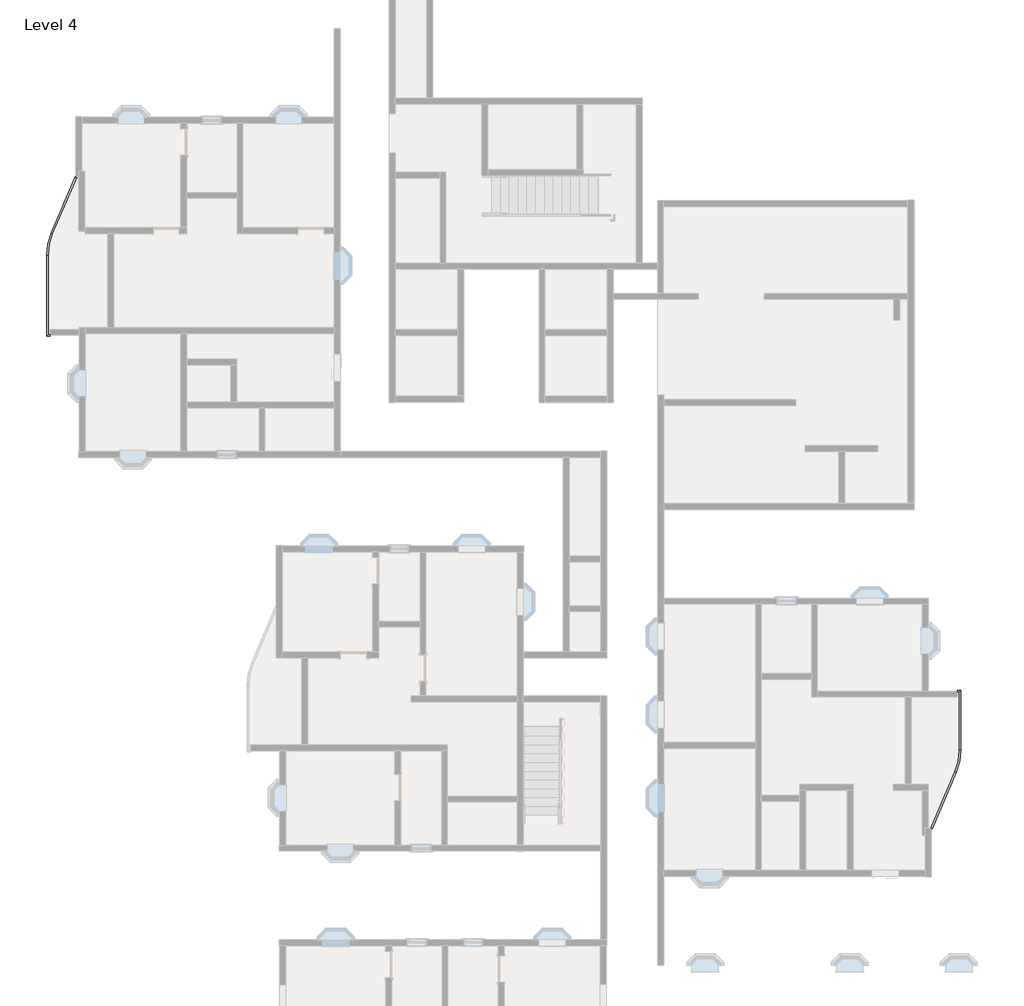
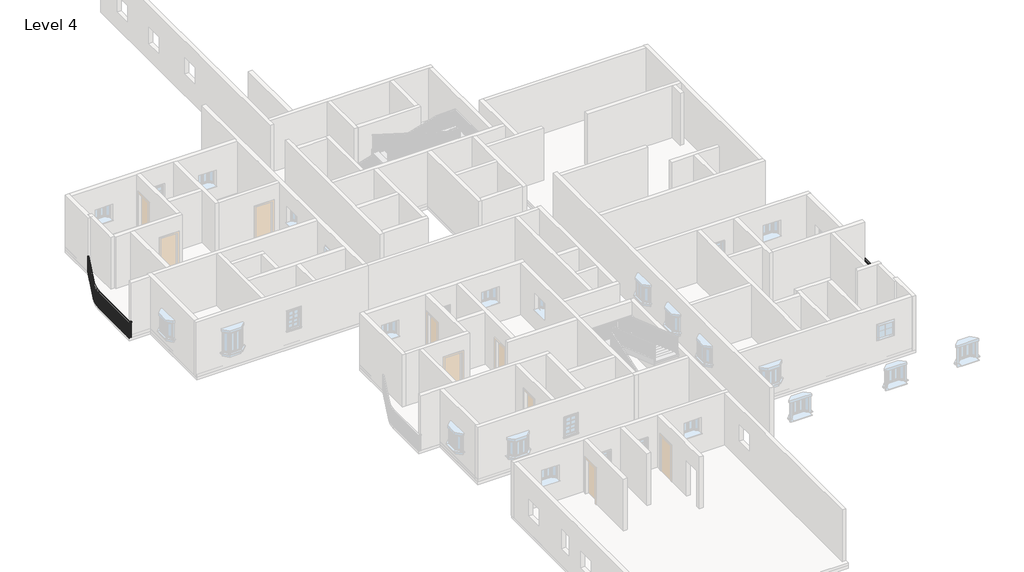
# One storey, part 9 of 14: 2 railings.
"""IFC4 building model written with IfcOpenShell, lengths in millimetres."""

from ifc_helpers import new_model, si_unit, frame, origin, place, context, project, spatial, polyline, circle_curve, outline, extrude, element, save
from ifc_brep_helpers import plane_surface, cylinder_surface, revolved_surface, advanced_brep

model = new_model("IFC4")

# Units and contexts
model_context = context("Model", 3, world=origin())
ifc_project = project(units=[si_unit("LENGTHUNIT", "METRE", prefix="MILLI")], contexts=[model_context])

# Site, building, storey
site = spatial("IfcSite", under=ifc_project)
building = spatial("IfcBuilding", under=site)
storey = spatial("IfcBuildingStorey", under=building, Name="Level 4", Elevation=9144.0)

# Railings
placement = place(None, origin())
element("IfcRailing", 1, ObjectType="Handrail - Rectangular", at=placement, inside=storey, context=model_context, shape_type="SolidModel", body=[
    advanced_brep(
    [(-19327.739878, 12446.0257339, 10058.4), (-19327.739878, 12446.0257339, 10007.6), (-19374.4383922, 12466.022953, 10007.6), (-19374.4383922, 12466.022953, 10058.4), (-20162.483418, 10496.6905323, 10058.4), (-20162.483418, 10496.6905323, 10007.6), (-20209.1819322, 10516.6877514, 10007.6), (-20209.1819322, 10516.6877514, 10058.4), (-20316.2891351, 9746.7948172, 10007.6), (-20316.2891351, 9746.7948172, 10058.4), (-20367.0891351, 9746.7948172, 10007.6), (-20367.0891351, 9746.7948172, 10058.4), (-20316.2891351, 7005.2583494, 10058.4), (-20316.2891351, 7005.2583494, 10007.6), (-20367.0891351, 6954.4583494, 10007.6), (-20367.0891351, 6954.4583494, 10058.4), (-20240.0891351, 7005.2583494, 10058.4), (-20240.0891351, 6954.4583494, 10058.4), (-20240.0891351, 6954.4583494, 10007.6), (-20240.0891351, 7005.2583494, 10007.6)],
    [
        (0, 1),
        (1, 2),
        (2, 3),
        (3, 0),
        (0, 4),
        (4, 5),
        (5, 1),
        (5, 6),
        (6, 2),
        (6, 7),
        (7, 3),
        (7, 4),
        (8, 5, circle_curve(frame((-18411.2891351, 9746.7948172, 10007.6), z_axis=(0.0, 0.0, -1.0), x_axis=(-0.919262090762392, 0.3936460446735823, 0.0)), 1905.0)),
        (4, 9, circle_curve(frame((-18411.2891351, 9746.7948172, 10058.4), z_axis=(0.0, 0.0, 1.0), x_axis=(-0.919262090762392, 0.3936460446735823, 0.0)), 1905.0)),
        (9, 8),
        (10, 6, circle_curve(frame((-18411.2891351, 9746.7948172, 10007.6), z_axis=(0.0, 0.0, -1.0), x_axis=(-0.919262090762392, 0.3936460446735823, 0.0)), 1955.8)),
        (8, 10),
        (11, 7, circle_curve(frame((-18411.2891351, 9746.7948172, 10058.4), z_axis=(0.0, 0.0, -1.0), x_axis=(-0.919262090762392, 0.3936460446735823, 0.0)), 1955.8)),
        (10, 11),
        (11, 9),
        (9, 12),
        (12, 13),
        (13, 8),
        (13, 14),
        (14, 10),
        (14, 15),
        (15, 11),
        (15, 12),
        (16, 17),
        (17, 18),
        (18, 19),
        (19, 16),
        (12, 16),
        (19, 13),
        (18, 14),
        (17, 15),
    ],
    [
        plane_surface(frame((-19351.0891351, 12456.0243434, 10058.4), z_axis=(0.3936460446735829, 0.9192620907623917, 0.0), x_axis=(0.9192620907623917, -0.3936460446735829, 0.0))),
        plane_surface(frame((-19327.739878, 12446.0257339, 10058.4), z_axis=(0.9192620907623915, -0.3936460446735834, 0.0), x_axis=(-0.3936460446735834, -0.9192620907623915, 0.0))),
        plane_surface(frame((-19327.739878, 12446.0257339, 10007.6), z_axis=(0.0, 0.0, -1.0000000000000002), x_axis=(-0.3936460446735834, -0.9192620907623915, 0.0))),
        plane_surface(frame((-19374.4383922, 12466.022953, 10007.6), z_axis=(-0.9192620907623916, 0.393646044673583, 0.0), x_axis=(-0.393646044673583, -0.9192620907623916, 0.0))),
        plane_surface(frame((-19374.4383922, 12466.022953, 10058.4), z_axis=(0.0, 0.0, 1.0), x_axis=(-0.393646044673583, -0.9192620907623916, 0.0))),
        revolved_surface(polyline([(-20162.483418002357, 10496.690532303173, 10058.4), (-20162.483418002357, 10496.690532303173, 10007.6)]), (-18411.2891351, 9746.7948172, 10058.4), (0.0, 0.0, 1.0)),
        plane_surface(frame((-18411.2891351, 9746.7948172, 10007.6), z_axis=(0.0, 0.0, -1.0), x_axis=(-0.919262090762392, 0.3936460446735823, 0.0))),
        cylinder_surface(frame((-18411.2891351, 9746.7948172, 10058.4), z_axis=(0.0, 0.0, 1.0), x_axis=(-0.919262090762392, 0.3936460446735823, 0.0)), 1955.8),
        plane_surface(frame((-18411.2891351, 9746.7948172, 10058.4), z_axis=(0.0, 0.0, 1.0), x_axis=(-0.919262090762392, 0.3936460446735823, 0.0))),
        plane_surface(frame((-20316.2891351, 9746.7948172, 10058.4), z_axis=(1.0, 0.0, 0.0), x_axis=(0.0, -1.0, 0.0))),
        plane_surface(frame((-20316.2891351, 9746.7948172, 10007.6), z_axis=(0.0, 0.0, -1.0), x_axis=(0.0, -1.0, 0.0))),
        plane_surface(frame((-20367.0891351, 9746.7948172, 10007.6), z_axis=(-1.0, 0.0, 0.0), x_axis=(0.0, -1.0, 0.0))),
        plane_surface(frame((-20367.0891351, 9746.7948172, 10058.4), z_axis=(0.0, 0.0, 1.0), x_axis=(0.0, -1.0, 0.0))),
        plane_surface(frame((-20240.0891351, 6979.8583494, 10058.4), z_axis=(1.0, 0.0, 0.0), x_axis=(0.0, 1.0, 0.0))),
        plane_surface(frame((-20316.2891351, 7005.2583494, 10058.4), z_axis=(0.0, 1.0, 0.0), x_axis=(1.0, 0.0, 0.0))),
        plane_surface(frame((-20316.2891351, 7005.2583494, 10007.6), z_axis=(0.0, 0.0, -1.0), x_axis=(1.0, 0.0, 0.0))),
        plane_surface(frame((-20367.0891351, 6954.4583494, 10007.6), z_axis=(0.0, -1.0, 0.0), x_axis=(1.0, 0.0, 0.0))),
        plane_surface(frame((-20367.0891351, 6954.4583494, 10058.4), z_axis=(0.0, 0.0, 1.0), x_axis=(1.0, 0.0, 0.0))),
    ],
    [
        (0, [[1, 2, 3, 4]]),
        (1, [[-1, 5, 6, 7]]),
        (2, [[-2, -7, 8, 9]]),
        (3, [[-3, -9, 10, 11]]),
        (4, [[-4, -11, 12, -5]]),
        (5, [[13, -6, 14, 15]]),
        (6, [[16, -8, -13, 17]]),
        (7, [[18, -10, -16, 19]]),
        (8, [[-14, -12, -18, 20]]),
        (9, [[-15, 21, 22, 23]]),
        (10, [[-17, -23, 24, 25]]),
        (11, [[-19, -25, 26, 27]]),
        (12, [[-20, -27, 28, -21]]),
        (13, [[29, 30, 31, 32]]),
        (14, [[-22, 33, -32, 34]]),
        (15, [[-24, -34, -31, 35]]),
        (16, [[-26, -35, -30, 36]]),
        (17, [[-28, -36, -29, -33]]),
    ],
),
    extrude(outline(polyline([(-20351.2141351, 7013.1198172), (-20332.1641351, 7013.1198172), (-20332.1641351, 6994.0698172), (-20351.2141351, 6994.0698172), (-20351.2141351, 7013.1198172)])), frame((0.0, 0.0, 9144.0), z_axis=(0.0, 0.0, 1.0), x_axis=(1.0, 0.0, 0.0)), (0.0, 0.0, 1.0), 863.6),
    extrude(outline(polyline([(-20351.2141351, 7114.7198172), (-20332.1641351, 7114.7198172), (-20332.1641351, 7095.6698172), (-20351.2141351, 7095.6698172), (-20351.2141351, 7114.7198172)])), frame((0.0, 0.0, 9144.0), z_axis=(0.0, 0.0, 1.0), x_axis=(1.0, 0.0, 0.0)), (0.0, 0.0, 1.0), 863.6),
    extrude(outline(polyline([(-20351.2141351, 7216.3198172), (-20332.1641351, 7216.3198172), (-20332.1641351, 7197.2698172), (-20351.2141351, 7197.2698172), (-20351.2141351, 7216.3198172)])), frame((0.0, 0.0, 9144.0), z_axis=(0.0, 0.0, 1.0), x_axis=(1.0, 0.0, 0.0)), (0.0, 0.0, 1.0), 863.6),
    extrude(outline(polyline([(-20351.2141351, 7317.9198172), (-20332.1641351, 7317.9198172), (-20332.1641351, 7298.8698172), (-20351.2141351, 7298.8698172), (-20351.2141351, 7317.9198172)])), frame((0.0, 0.0, 9144.0), z_axis=(0.0, 0.0, 1.0), x_axis=(1.0, 0.0, 0.0)), (0.0, 0.0, 1.0), 863.6),
    extrude(outline(polyline([(-20351.2141351, 7419.5198172), (-20332.1641351, 7419.5198172), (-20332.1641351, 7400.4698172), (-20351.2141351, 7400.4698172), (-20351.2141351, 7419.5198172)])), frame((0.0, 0.0, 9144.0), z_axis=(0.0, 0.0, 1.0), x_axis=(1.0, 0.0, 0.0)), (0.0, 0.0, 1.0), 863.6),
    extrude(outline(polyline([(-20351.2141351, 7521.1198172), (-20332.1641351, 7521.1198172), (-20332.1641351, 7502.0698172), (-20351.2141351, 7502.0698172), (-20351.2141351, 7521.1198172)])), frame((0.0, 0.0, 9144.0), z_axis=(0.0, 0.0, 1.0), x_axis=(1.0, 0.0, 0.0)), (0.0, 0.0, 1.0), 863.6),
    extrude(outline(polyline([(-20351.2141351, 7622.7198172), (-20332.1641351, 7622.7198172), (-20332.1641351, 7603.6698172), (-20351.2141351, 7603.6698172), (-20351.2141351, 7622.7198172)])), frame((0.0, 0.0, 9144.0), z_axis=(0.0, 0.0, 1.0), x_axis=(1.0, 0.0, 0.0)), (0.0, 0.0, 1.0), 863.6),
    extrude(outline(polyline([(-20351.2141351, 7724.3198172), (-20332.1641351, 7724.3198172), (-20332.1641351, 7705.2698172), (-20351.2141351, 7705.2698172), (-20351.2141351, 7724.3198172)])), frame((0.0, 0.0, 9144.0), z_axis=(0.0, 0.0, 1.0), x_axis=(1.0, 0.0, 0.0)), (0.0, 0.0, 1.0), 863.6),
    extrude(outline(polyline([(-20351.2141351, 7825.9198172), (-20332.1641351, 7825.9198172), (-20332.1641351, 7806.8698172), (-20351.2141351, 7806.8698172), (-20351.2141351, 7825.9198172)])), frame((0.0, 0.0, 9144.0), z_axis=(0.0, 0.0, 1.0), x_axis=(1.0, 0.0, 0.0)), (0.0, 0.0, 1.0), 863.6),
    extrude(outline(polyline([(-20351.2141351, 7927.5198172), (-20332.1641351, 7927.5198172), (-20332.1641351, 7908.4698172), (-20351.2141351, 7908.4698172), (-20351.2141351, 7927.5198172)])), frame((0.0, 0.0, 9144.0), z_axis=(0.0, 0.0, 1.0), x_axis=(1.0, 0.0, 0.0)), (0.0, 0.0, 1.0), 863.6),
    extrude(outline(polyline([(-20351.2141351, 8029.1198172), (-20332.1641351, 8029.1198172), (-20332.1641351, 8010.0698172), (-20351.2141351, 8010.0698172), (-20351.2141351, 8029.1198172)])), frame((0.0, 0.0, 9144.0), z_axis=(0.0, 0.0, 1.0), x_axis=(1.0, 0.0, 0.0)), (0.0, 0.0, 1.0), 863.6),
    extrude(outline(polyline([(-20351.2141351, 8130.7198172), (-20332.1641351, 8130.7198172), (-20332.1641351, 8111.6698172), (-20351.2141351, 8111.6698172), (-20351.2141351, 8130.7198172)])), frame((0.0, 0.0, 9144.0), z_axis=(0.0, 0.0, 1.0), x_axis=(1.0, 0.0, 0.0)), (0.0, 0.0, 1.0), 863.6),
    extrude(outline(polyline([(-20351.2141351, 8232.3198172), (-20332.1641351, 8232.3198172), (-20332.1641351, 8213.2698172), (-20351.2141351, 8213.2698172), (-20351.2141351, 8232.3198172)])), frame((0.0, 0.0, 9144.0), z_axis=(0.0, 0.0, 1.0), x_axis=(1.0, 0.0, 0.0)), (0.0, 0.0, 1.0), 863.6),
    extrude(outline(polyline([(-20351.2141351, 8333.9198172), (-20332.1641351, 8333.9198172), (-20332.1641351, 8314.8698172), (-20351.2141351, 8314.8698172), (-20351.2141351, 8333.9198172)])), frame((0.0, 0.0, 9144.0), z_axis=(0.0, 0.0, 1.0), x_axis=(1.0, 0.0, 0.0)), (0.0, 0.0, 1.0), 863.6),
    extrude(outline(polyline([(-20351.2141351, 8435.5198172), (-20332.1641351, 8435.5198172), (-20332.1641351, 8416.4698172), (-20351.2141351, 8416.4698172), (-20351.2141351, 8435.5198172)])), frame((0.0, 0.0, 9144.0), z_axis=(0.0, 0.0, 1.0), x_axis=(1.0, 0.0, 0.0)), (0.0, 0.0, 1.0), 863.6),
    extrude(outline(polyline([(-20351.2141351, 8537.1198172), (-20332.1641351, 8537.1198172), (-20332.1641351, 8518.0698172), (-20351.2141351, 8518.0698172), (-20351.2141351, 8537.1198172)])), frame((0.0, 0.0, 9144.0), z_axis=(0.0, 0.0, 1.0), x_axis=(1.0, 0.0, 0.0)), (0.0, 0.0, 1.0), 863.6),
    extrude(outline(polyline([(-20351.2141351, 8638.7198172), (-20332.1641351, 8638.7198172), (-20332.1641351, 8619.6698172), (-20351.2141351, 8619.6698172), (-20351.2141351, 8638.7198172)])), frame((0.0, 0.0, 9144.0), z_axis=(0.0, 0.0, 1.0), x_axis=(1.0, 0.0, 0.0)), (0.0, 0.0, 1.0), 863.6),
    extrude(outline(polyline([(-20351.2141351, 8740.3198172), (-20332.1641351, 8740.3198172), (-20332.1641351, 8721.2698172), (-20351.2141351, 8721.2698172), (-20351.2141351, 8740.3198172)])), frame((0.0, 0.0, 9144.0), z_axis=(0.0, 0.0, 1.0), x_axis=(1.0, 0.0, 0.0)), (0.0, 0.0, 1.0), 863.6),
    extrude(outline(polyline([(-20351.2141351, 8841.9198172), (-20332.1641351, 8841.9198172), (-20332.1641351, 8822.8698172), (-20351.2141351, 8822.8698172), (-20351.2141351, 8841.9198172)])), frame((0.0, 0.0, 9144.0), z_axis=(0.0, 0.0, 1.0), x_axis=(1.0, 0.0, 0.0)), (0.0, 0.0, 1.0), 863.6),
    extrude(outline(polyline([(-20351.2141351, 8943.5198172), (-20332.1641351, 8943.5198172), (-20332.1641351, 8924.4698172), (-20351.2141351, 8924.4698172), (-20351.2141351, 8943.5198172)])), frame((0.0, 0.0, 9144.0), z_axis=(0.0, 0.0, 1.0), x_axis=(1.0, 0.0, 0.0)), (0.0, 0.0, 1.0), 863.6),
    extrude(outline(polyline([(-20351.2141351, 9045.1198172), (-20332.1641351, 9045.1198172), (-20332.1641351, 9026.0698172), (-20351.2141351, 9026.0698172), (-20351.2141351, 9045.1198172)])), frame((0.0, 0.0, 9144.0), z_axis=(0.0, 0.0, 1.0), x_axis=(1.0, 0.0, 0.0)), (0.0, 0.0, 1.0), 863.6),
    extrude(outline(polyline([(-20351.2141351, 9146.7198172), (-20332.1641351, 9146.7198172), (-20332.1641351, 9127.6698172), (-20351.2141351, 9127.6698172), (-20351.2141351, 9146.7198172)])), frame((0.0, 0.0, 9144.0), z_axis=(0.0, 0.0, 1.0), x_axis=(1.0, 0.0, 0.0)), (0.0, 0.0, 1.0), 863.6),
    extrude(outline(polyline([(-20351.2141351, 9248.3198172), (-20332.1641351, 9248.3198172), (-20332.1641351, 9229.2698172), (-20351.2141351, 9229.2698172), (-20351.2141351, 9248.3198172)])), frame((0.0, 0.0, 9144.0), z_axis=(0.0, 0.0, 1.0), x_axis=(1.0, 0.0, 0.0)), (0.0, 0.0, 1.0), 863.6),
    extrude(outline(polyline([(-20351.2141351, 9349.9198172), (-20332.1641351, 9349.9198172), (-20332.1641351, 9330.8698172), (-20351.2141351, 9330.8698172), (-20351.2141351, 9349.9198172)])), frame((0.0, 0.0, 9144.0), z_axis=(0.0, 0.0, 1.0), x_axis=(1.0, 0.0, 0.0)), (0.0, 0.0, 1.0), 863.6),
    extrude(outline(polyline([(-20351.2141351, 9451.5198172), (-20332.1641351, 9451.5198172), (-20332.1641351, 9432.4698172), (-20351.2141351, 9432.4698172), (-20351.2141351, 9451.5198172)])), frame((0.0, 0.0, 9144.0), z_axis=(0.0, 0.0, 1.0), x_axis=(1.0, 0.0, 0.0)), (0.0, 0.0, 1.0), 863.6),
    extrude(outline(polyline([(-20351.2141351, 9553.1198172), (-20332.1641351, 9553.1198172), (-20332.1641351, 9534.0698172), (-20351.2141351, 9534.0698172), (-20351.2141351, 9553.1198172)])), frame((0.0, 0.0, 9144.0), z_axis=(0.0, 0.0, 1.0), x_axis=(1.0, 0.0, 0.0)), (0.0, 0.0, 1.0), 863.6),
    extrude(outline(polyline([(-20351.2141351, 9654.7198172), (-20332.1641351, 9654.7198172), (-20332.1641351, 9635.6698172), (-20351.2141351, 9635.6698172), (-20351.2141351, 9654.7198172)])), frame((0.0, 0.0, 9144.0), z_axis=(0.0, 0.0, 1.0), x_axis=(1.0, 0.0, 0.0)), (0.0, 0.0, 1.0), 863.6),
    extrude(outline(polyline([(-20349.6005818, 9826.4720848), (-20330.5630441, 9825.7831307), (-20331.2519982, 9806.745593), (-20350.289536, 9807.4345471), (-20349.6005818, 9826.4720848)])), frame((0.0, 0.0, 9144.0), z_axis=(0.0, 0.0, 1.0), x_axis=(1.0, 0.0, 0.0)), (0.0, 0.0, 1.0), 863.6),
    extrude(outline(polyline([(-20342.724955, 9928.3310534), (-20323.750023, 9926.6415402), (-20325.4395363, 9907.6666081), (-20344.4144683, 9909.3561214), (-20342.724955, 9928.3310534)])), frame((0.0, 0.0, 9144.0), z_axis=(0.0, 0.0, 1.0), x_axis=(1.0, 0.0, 0.0)), (0.0, 0.0, 1.0), 863.6),
    extrude(outline(polyline([(-20330.5003254, 10029.6872677), (-20311.6405491, 10027.0018743), (-20314.3259425, 10008.142098), (-20333.1857188, 10010.8274914), (-20330.5003254, 10029.6872677)])), frame((0.0, 0.0, 9144.0), z_axis=(0.0, 0.0, 1.0), x_axis=(1.0, 0.0, 0.0)), (0.0, 0.0, 1.0), 863.6),
    extrude(outline(polyline([(-20312.9605484, 10130.2600272), (-20294.2681589, 10126.5861907), (-20297.9419954, 10107.8938012), (-20316.6343849, 10111.5676377), (-20312.9605484, 10130.2600272)])), frame((0.0, 0.0, 9144.0), z_axis=(0.0, 0.0, 1.0), x_axis=(1.0, 0.0, 0.0)), (0.0, 0.0, 1.0), 863.6),
    extrude(outline(polyline([(-20290.1541995, 10229.7708014), (-20271.6809643, 10225.1186963), (-20276.3330693, 10206.6454611), (-20294.8063045, 10211.2975662), (-20290.1541995, 10229.7708014)])), frame((0.0, 0.0, 9144.0), z_axis=(0.0, 0.0, 1.0), x_axis=(1.0, 0.0, 0.0)), (0.0, 0.0, 1.0), 863.6),
    extrude(outline(polyline([(-20262.1444395, 10327.9440008), (-20243.9415192, 10322.3265109), (-20249.5590091, 10304.1235906), (-20267.7619294, 10309.7410805), (-20262.1444395, 10327.9440008)])), frame((0.0, 0.0, 9144.0), z_axis=(0.0, 0.0, 1.0), x_axis=(1.0, 0.0, 0.0)), (0.0, 0.0, 1.0), 863.6),
    extrude(outline(polyline([(-20229.0088399, 10424.5077402), (-20211.1266465, 10417.9404228), (-20217.693964, 10400.0582293), (-20235.5761574, 10406.6255468), (-20229.0088399, 10424.5077402)])), frame((0.0, 0.0, 9144.0), z_axis=(0.0, 0.0, 1.0), x_axis=(1.0, 0.0, 0.0)), (0.0, 0.0, 1.0), 863.6),
    extrude(outline(polyline([(-20155.9843907, 10600.589225), (-20138.4724479, 10593.0902678), (-20145.9714051, 10575.578325), (-20163.4833479, 10583.0772822), (-20155.9843907, 10600.589225)])), frame((0.0, 0.0, 9144.0), z_axis=(0.0, 0.0, 1.0), x_axis=(1.0, 0.0, 0.0)), (0.0, 0.0, 1.0), 863.6),
    extrude(outline(polyline([(-20115.9899526, 10693.9862534), (-20098.4780098, 10686.4872963), (-20105.9769669, 10668.9753534), (-20123.4889098, 10676.4743106), (-20115.9899526, 10693.9862534)])), frame((0.0, 0.0, 9144.0), z_axis=(0.0, 0.0, 1.0), x_axis=(1.0, 0.0, 0.0)), (0.0, 0.0, 1.0), 863.6),
    extrude(outline(polyline([(-20075.9955145, 10787.3832818), (-20058.4835716, 10779.8843247), (-20065.9825288, 10762.3723818), (-20083.4944716, 10769.871339), (-20075.9955145, 10787.3832818)])), frame((0.0, 0.0, 9144.0), z_axis=(0.0, 0.0, 1.0), x_axis=(1.0, 0.0, 0.0)), (0.0, 0.0, 1.0), 863.6),
    extrude(outline(polyline([(-20036.0010763, 10880.7803103), (-20018.4891335, 10873.2813531), (-20025.9880906, 10855.7694103), (-20043.5000335, 10863.2683674), (-20036.0010763, 10880.7803103)])), frame((0.0, 0.0, 9144.0), z_axis=(0.0, 0.0, 1.0), x_axis=(1.0, 0.0, 0.0)), (0.0, 0.0, 1.0), 863.6),
    extrude(outline(polyline([(-19996.0066382, 10974.1773387), (-19978.4946954, 10966.6783815), (-19985.9936525, 10949.1664387), (-20003.5055953, 10956.6653958), (-19996.0066382, 10974.1773387)])), frame((0.0, 0.0, 9144.0), z_axis=(0.0, 0.0, 1.0), x_axis=(1.0, 0.0, 0.0)), (0.0, 0.0, 1.0), 863.6),
    extrude(outline(polyline([(-19956.0122, 11067.5743671), (-19938.5002572, 11060.0754099), (-19945.9992144, 11042.5634671), (-19963.5111572, 11050.0624243), (-19956.0122, 11067.5743671)])), frame((0.0, 0.0, 9144.0), z_axis=(0.0, 0.0, 1.0), x_axis=(1.0, 0.0, 0.0)), (0.0, 0.0, 1.0), 863.6),
    extrude(outline(polyline([(-19916.0177619, 11160.9713955), (-19898.5058191, 11153.4724384), (-19906.0047762, 11135.9604955), (-19923.5167191, 11143.4594527), (-19916.0177619, 11160.9713955)])), frame((0.0, 0.0, 9144.0), z_axis=(0.0, 0.0, 1.0), x_axis=(1.0, 0.0, 0.0)), (0.0, 0.0, 1.0), 863.6),
    extrude(outline(polyline([(-19876.0233238, 11254.3684239), (-19858.5113809, 11246.8694668), (-19866.0103381, 11229.357524), (-19883.5222809, 11236.8564811), (-19876.0233238, 11254.3684239)])), frame((0.0, 0.0, 9144.0), z_axis=(0.0, 0.0, 1.0), x_axis=(1.0, 0.0, 0.0)), (0.0, 0.0, 1.0), 863.6),
    extrude(outline(polyline([(-19836.0288856, 11347.7654524), (-19818.5169428, 11340.2664952), (-19826.0159, 11322.7545524), (-19843.5278428, 11330.2535095), (-19836.0288856, 11347.7654524)])), frame((0.0, 0.0, 9144.0), z_axis=(0.0, 0.0, 1.0), x_axis=(1.0, 0.0, 0.0)), (0.0, 0.0, 1.0), 863.6),
    extrude(outline(polyline([(-19796.0344475, 11441.1624808), (-19778.5225047, 11433.6635236), (-19786.0214618, 11416.1515808), (-19803.5334046, 11423.650538), (-19796.0344475, 11441.1624808)])), frame((0.0, 0.0, 9144.0), z_axis=(0.0, 0.0, 1.0), x_axis=(1.0, 0.0, 0.0)), (0.0, 0.0, 1.0), 863.6),
    extrude(outline(polyline([(-19756.0400094, 11534.5595092), (-19738.5280665, 11527.060552), (-19746.0270237, 11509.5486092), (-19763.5389665, 11517.0475664), (-19756.0400094, 11534.5595092)])), frame((0.0, 0.0, 9144.0), z_axis=(0.0, 0.0, 1.0), x_axis=(1.0, 0.0, 0.0)), (0.0, 0.0, 1.0), 863.6),
    extrude(outline(polyline([(-19716.0455712, 11627.9565376), (-19698.5336284, 11620.4575805), (-19706.0325855, 11602.9456376), (-19723.5445284, 11610.4445948), (-19716.0455712, 11627.9565376)])), frame((0.0, 0.0, 9144.0), z_axis=(0.0, 0.0, 1.0), x_axis=(1.0, 0.0, 0.0)), (0.0, 0.0, 1.0), 863.6),
    extrude(outline(polyline([(-19676.0511331, 11721.353566), (-19658.5391902, 11713.8546089), (-19666.0381474, 11696.3426661), (-19683.5500902, 11703.8416232), (-19676.0511331, 11721.353566)])), frame((0.0, 0.0, 9144.0), z_axis=(0.0, 0.0, 1.0), x_axis=(1.0, 0.0, 0.0)), (0.0, 0.0, 1.0), 863.6),
    extrude(outline(polyline([(-19636.0566949, 11814.7505945), (-19618.5447521, 11807.2516373), (-19626.0437093, 11789.7396945), (-19643.5556521, 11797.2386516), (-19636.0566949, 11814.7505945)])), frame((0.0, 0.0, 9144.0), z_axis=(0.0, 0.0, 1.0), x_axis=(1.0, 0.0, 0.0)), (0.0, 0.0, 1.0), 863.6),
    extrude(outline(polyline([(-19596.0622568, 11908.1476229), (-19578.550314, 11900.6486657), (-19586.0492711, 11883.1367229), (-19603.561214, 11890.6356801), (-19596.0622568, 11908.1476229)])), frame((0.0, 0.0, 9144.0), z_axis=(0.0, 0.0, 1.0), x_axis=(1.0, 0.0, 0.0)), (0.0, 0.0, 1.0), 863.6),
    extrude(outline(polyline([(-19556.0678187, 12001.5446513), (-19538.5558758, 11994.0456942), (-19546.054833, 11976.5337513), (-19563.5667758, 11984.0327085), (-19556.0678187, 12001.5446513)])), frame((0.0, 0.0, 9144.0), z_axis=(0.0, 0.0, 1.0), x_axis=(1.0, 0.0, 0.0)), (0.0, 0.0, 1.0), 863.6),
    extrude(outline(polyline([(-19516.0733805, 12094.9416797), (-19498.5614377, 12087.4427226), (-19506.0603948, 12069.9307797), (-19523.5723377, 12077.4297369), (-19516.0733805, 12094.9416797)])), frame((0.0, 0.0, 9144.0), z_axis=(0.0, 0.0, 1.0), x_axis=(1.0, 0.0, 0.0)), (0.0, 0.0, 1.0), 863.6),
    extrude(outline(polyline([(-19476.0789424, 12188.3387082), (-19458.5669996, 12180.839751), (-19466.0659567, 12163.3278082), (-19483.5778995, 12170.8267653), (-19476.0789424, 12188.3387082)])), frame((0.0, 0.0, 9144.0), z_axis=(0.0, 0.0, 1.0), x_axis=(1.0, 0.0, 0.0)), (0.0, 0.0, 1.0), 863.6),
    extrude(outline(polyline([(-19436.0845042, 12281.7357366), (-19418.5725614, 12274.2367794), (-19426.0715186, 12256.7248366), (-19443.5834614, 12264.2237937), (-19436.0845042, 12281.7357366)])), frame((0.0, 0.0, 9144.0), z_axis=(0.0, 0.0, 1.0), x_axis=(1.0, 0.0, 0.0)), (0.0, 0.0, 1.0), 863.6),
    extrude(outline(polyline([(-19396.0900661, 12375.132765), (-19378.5781233, 12367.6338078), (-19386.0770804, 12350.121865), (-19403.5890233, 12357.6208222), (-19396.0900661, 12375.132765)])), frame((0.0, 0.0, 9144.0), z_axis=(0.0, 0.0, 1.0), x_axis=(1.0, 0.0, 0.0)), (0.0, 0.0, 1.0), 863.6),
    extrude(outline(polyline([(-20351.2141351, 6989.3833494), (-20332.1641351, 6989.3833494), (-20332.1641351, 6970.3333494), (-20351.2141351, 6970.3333494), (-20351.2141351, 6989.3833494)])), frame((0.0, 0.0, 9144.0), z_axis=(0.0, 0.0, 1.0), x_axis=(1.0, 0.0, 0.0)), (0.0, 0.0, 1.0), 863.6),
    extrude(outline(polyline([(-20351.2141351, 9756.3198172), (-20332.1641351, 9756.3198172), (-20332.1641351, 9737.2698172), (-20351.2141351, 9737.2698172), (-20351.2141351, 9756.3198172)])), frame((0.0, 0.0, 9144.0), z_axis=(0.0, 0.0, 1.0), x_axis=(1.0, 0.0, 0.0)), (0.0, 0.0, 1.0), 863.6),
    extrude(outline(polyline([(-20190.839168, 10519.1945919), (-20173.3272251, 10511.6956347), (-20180.8261823, 10494.1836919), (-20198.3381251, 10501.682649), (-20190.839168, 10519.1945919)])), frame((0.0, 0.0, 9144.0), z_axis=(0.0, 0.0, 1.0), x_axis=(1.0, 0.0, 0.0)), (0.0, 0.0, 1.0), 863.6),
    extrude(outline(polyline([(-20259.1391351, 6970.3333494), (-20259.1391351, 6989.3833494), (-20240.0891351, 6989.3833494), (-20240.0891351, 6970.3333494), (-20259.1391351, 6970.3333494)])), frame((0.0, 0.0, 9144.0), z_axis=(0.0, 0.0, 1.0), x_axis=(1.0, 0.0, 0.0)), (0.0, 0.0, 1.0), 863.6),
    extrude(outline(polyline([(-19359.8451065, 12459.773822), (-19342.3331637, 12452.2748648), (-19349.8321209, 12434.762922), (-19367.3440637, 12442.2618792), (-19359.8451065, 12459.773822)])), frame((0.0, 0.0, 9144.0), z_axis=(0.0, 0.0, 1.0), x_axis=(1.0, 0.0, 0.0)), (0.0, 0.0, 1.0), 863.6),
])
element("IfcRailing", 2, ObjectType="Handrail - Rectangular", at=placement, inside=storey, context=model_context, shape_type="SolidModel", body=[
    advanced_brep(
    [(10250.7887952, -10096.81198, 10058.4), (10250.7887952, -10096.81198, 10007.6), (10297.4873094, -10116.8091991, 10007.6), (10297.4873094, -10116.8091991, 10058.4), (11085.5323352, -8147.4767784, 10058.4), (11085.5323352, -8147.4767784, 10007.6), (11132.2308494, -8167.4739975, 10007.6), (11132.2308494, -8167.4739975, 10058.4), (11239.3380523, -7397.5810633, 10007.6), (11239.3380523, -7397.5810633, 10058.4), (11290.1380523, -7397.5810633, 10007.6), (11290.1380523, -7397.5810633, 10058.4), (11239.3380523, -5378.0542694, 10058.4), (11239.3380523, -5378.0542694, 10007.6), (11290.1380523, -5327.2542694, 10007.6), (11290.1380523, -5327.2542694, 10058.4), (11163.1380523, -5378.0542694, 10058.4), (11163.1380523, -5327.2542694, 10058.4), (11163.1380523, -5327.2542694, 10007.6), (11163.1380523, -5378.0542694, 10007.6)],
    [
        (0, 1),
        (1, 2),
        (2, 3),
        (3, 0),
        (0, 4),
        (4, 5),
        (5, 1),
        (5, 6),
        (6, 2),
        (6, 7),
        (7, 3),
        (7, 4),
        (8, 5, circle_curve(frame((9334.3380523, -7397.5810633, 10007.6), z_axis=(0.0, 0.0, -1.0), x_axis=(0.9192620907624003, -0.3936460446735628, 0.0)), 1905.0)),
        (4, 9, circle_curve(frame((9334.3380523, -7397.5810633, 10058.4), z_axis=(0.0, 0.0, 1.0), x_axis=(0.9192620907624003, -0.3936460446735628, 0.0)), 1905.0)),
        (9, 8),
        (10, 6, circle_curve(frame((9334.3380523, -7397.5810633, 10007.6), z_axis=(0.0, 0.0, -1.0), x_axis=(0.9192620907624003, -0.3936460446735628, 0.0)), 1955.8)),
        (8, 10),
        (11, 7, circle_curve(frame((9334.3380523, -7397.5810633, 10058.4), z_axis=(0.0, 0.0, -1.0), x_axis=(0.9192620907624003, -0.3936460446735628, 0.0)), 1955.8)),
        (10, 11),
        (11, 9),
        (9, 12),
        (12, 13),
        (13, 8),
        (13, 14),
        (14, 10),
        (14, 15),
        (15, 11),
        (15, 12),
        (16, 17),
        (17, 18),
        (18, 19),
        (19, 16),
        (12, 16),
        (19, 13),
        (18, 14),
        (17, 15),
    ],
    [
        plane_surface(frame((10274.1380523, -10106.8105895, 10058.4), z_axis=(-0.3936460446735629, -0.9192620907624003, 0.0), x_axis=(0.9192620907624003, -0.3936460446735629, 0.0))),
        plane_surface(frame((10250.7887952, -10096.81198, 10058.4), z_axis=(-0.9192620907624005, 0.39364604467356235, 0.0), x_axis=(0.39364604467356235, 0.9192620907624005, 0.0))),
        plane_surface(frame((10250.7887952, -10096.81198, 10007.6), z_axis=(0.0, 0.0, -1.0), x_axis=(0.39364604467356235, 0.9192620907624005, 0.0))),
        plane_surface(frame((10297.4873094, -10116.8091991, 10007.6), z_axis=(0.9192620907624003, -0.3936460446735627, 0.0), x_axis=(0.3936460446735627, 0.9192620907624003, 0.0))),
        plane_surface(frame((10297.4873094, -10116.8091991, 10058.4), z_axis=(0.0, 0.0, 1.0), x_axis=(0.3936460446735627, 0.9192620907624003, 0.0))),
        revolved_surface(polyline([(11085.532335202372, -8147.476778403137, 10058.4), (11085.532335202372, -8147.476778403137, 10007.6)]), (9334.3380523, -7397.5810633, 10058.4), (0.0, 0.0, 1.0)),
        plane_surface(frame((9334.3380523, -7397.5810633, 10007.6), z_axis=(0.0, 0.0, -1.0), x_axis=(0.9192620907624003, -0.3936460446735628, 0.0))),
        cylinder_surface(frame((9334.3380523, -7397.5810633, 10058.4), z_axis=(0.0, 0.0, 1.0), x_axis=(0.9192620907624003, -0.3936460446735628, 0.0)), 1955.8),
        plane_surface(frame((9334.3380523, -7397.5810633, 10058.4), z_axis=(0.0, 0.0, 1.0), x_axis=(0.9192620907624003, -0.3936460446735628, 0.0))),
        plane_surface(frame((11239.3380523, -7397.5810633, 10058.4), z_axis=(-1.0, 0.0, 0.0), x_axis=(0.0, 1.0, 0.0))),
        plane_surface(frame((11239.3380523, -7397.5810633, 10007.6), z_axis=(0.0, 0.0, -1.0), x_axis=(0.0, 1.0, 0.0))),
        plane_surface(frame((11290.1380523, -7397.5810633, 10007.6), z_axis=(1.0, 0.0, 0.0), x_axis=(0.0, 1.0, 0.0))),
        plane_surface(frame((11290.1380523, -7397.5810633, 10058.4), z_axis=(0.0, 0.0, 1.0), x_axis=(0.0, 1.0, 0.0))),
        plane_surface(frame((11163.1380523, -5352.6542694, 10058.4), z_axis=(-1.0, 0.0, 0.0), x_axis=(0.0, -1.0, 0.0))),
        plane_surface(frame((11239.3380523, -5378.0542694, 10058.4), z_axis=(0.0, -1.0, 0.0), x_axis=(-1.0, 0.0, 0.0))),
        plane_surface(frame((11239.3380523, -5378.0542694, 10007.6), z_axis=(0.0, 0.0, -1.0), x_axis=(-1.0, 0.0, 0.0))),
        plane_surface(frame((11290.1380523, -5327.2542694, 10007.6), z_axis=(0.0, 1.0, 0.0), x_axis=(-1.0, 0.0, 0.0))),
        plane_surface(frame((11290.1380523, -5327.2542694, 10058.4), z_axis=(0.0, 0.0, 1.0), x_axis=(-1.0, 0.0, 0.0))),
    ],
    [
        (0, [[1, 2, 3, 4]]),
        (1, [[-1, 5, 6, 7]]),
        (2, [[-2, -7, 8, 9]]),
        (3, [[-3, -9, 10, 11]]),
        (4, [[-4, -11, 12, -5]]),
        (5, [[13, -6, 14, 15]]),
        (6, [[16, -8, -13, 17]]),
        (7, [[18, -10, -16, 19]]),
        (8, [[-14, -12, -18, 20]]),
        (9, [[-15, 21, 22, 23]]),
        (10, [[-17, -23, 24, 25]]),
        (11, [[-19, -25, 26, 27]]),
        (12, [[-20, -27, 28, -21]]),
        (13, [[29, 30, 31, 32]]),
        (14, [[-22, 33, -32, 34]]),
        (15, [[-24, -34, -31, 35]]),
        (16, [[-26, -35, -30, 36]]),
        (17, [[-28, -36, -29, -33]]),
    ],
),
    extrude(outline(polyline([(11274.2630523, -5375.1060633), (11255.2130523, -5375.1060633), (11255.2130523, -5356.0560633), (11274.2630523, -5356.0560633), (11274.2630523, -5375.1060633)])), frame((0.0, 0.0, 9144.0), z_axis=(0.0, 0.0, 1.0), x_axis=(1.0, 0.0, 0.0)), (0.0, 0.0, 1.0), 863.6),
    extrude(outline(polyline([(11274.2630523, -5476.7060633), (11255.2130523, -5476.7060633), (11255.2130523, -5457.6560633), (11274.2630523, -5457.6560633), (11274.2630523, -5476.7060633)])), frame((0.0, 0.0, 9144.0), z_axis=(0.0, 0.0, 1.0), x_axis=(1.0, 0.0, 0.0)), (0.0, 0.0, 1.0), 863.6),
    extrude(outline(polyline([(11274.2630523, -5578.3060633), (11255.2130523, -5578.3060633), (11255.2130523, -5559.2560633), (11274.2630523, -5559.2560633), (11274.2630523, -5578.3060633)])), frame((0.0, 0.0, 9144.0), z_axis=(0.0, 0.0, 1.0), x_axis=(1.0, 0.0, 0.0)), (0.0, 0.0, 1.0), 863.6),
    extrude(outline(polyline([(11274.2630523, -5679.9060633), (11255.2130523, -5679.9060633), (11255.2130523, -5660.8560633), (11274.2630523, -5660.8560633), (11274.2630523, -5679.9060633)])), frame((0.0, 0.0, 9144.0), z_axis=(0.0, 0.0, 1.0), x_axis=(1.0, 0.0, 0.0)), (0.0, 0.0, 1.0), 863.6),
    extrude(outline(polyline([(11274.2630523, -5781.5060633), (11255.2130523, -5781.5060633), (11255.2130523, -5762.4560633), (11274.2630523, -5762.4560633), (11274.2630523, -5781.5060633)])), frame((0.0, 0.0, 9144.0), z_axis=(0.0, 0.0, 1.0), x_axis=(1.0, 0.0, 0.0)), (0.0, 0.0, 1.0), 863.6),
    extrude(outline(polyline([(11274.2630523, -5883.1060633), (11255.2130523, -5883.1060633), (11255.2130523, -5864.0560633), (11274.2630523, -5864.0560633), (11274.2630523, -5883.1060633)])), frame((0.0, 0.0, 9144.0), z_axis=(0.0, 0.0, 1.0), x_axis=(1.0, 0.0, 0.0)), (0.0, 0.0, 1.0), 863.6),
    extrude(outline(polyline([(11274.2630523, -5984.7060633), (11255.2130523, -5984.7060633), (11255.2130523, -5965.6560633), (11274.2630523, -5965.6560633), (11274.2630523, -5984.7060633)])), frame((0.0, 0.0, 9144.0), z_axis=(0.0, 0.0, 1.0), x_axis=(1.0, 0.0, 0.0)), (0.0, 0.0, 1.0), 863.6),
    extrude(outline(polyline([(11274.2630523, -6086.3060633), (11255.2130523, -6086.3060633), (11255.2130523, -6067.2560633), (11274.2630523, -6067.2560633), (11274.2630523, -6086.3060633)])), frame((0.0, 0.0, 9144.0), z_axis=(0.0, 0.0, 1.0), x_axis=(1.0, 0.0, 0.0)), (0.0, 0.0, 1.0), 863.6),
    extrude(outline(polyline([(11274.2630523, -6187.9060633), (11255.2130523, -6187.9060633), (11255.2130523, -6168.8560633), (11274.2630523, -6168.8560633), (11274.2630523, -6187.9060633)])), frame((0.0, 0.0, 9144.0), z_axis=(0.0, 0.0, 1.0), x_axis=(1.0, 0.0, 0.0)), (0.0, 0.0, 1.0), 863.6),
    extrude(outline(polyline([(11274.2630523, -6289.5060633), (11255.2130523, -6289.5060633), (11255.2130523, -6270.4560633), (11274.2630523, -6270.4560633), (11274.2630523, -6289.5060633)])), frame((0.0, 0.0, 9144.0), z_axis=(0.0, 0.0, 1.0), x_axis=(1.0, 0.0, 0.0)), (0.0, 0.0, 1.0), 863.6),
    extrude(outline(polyline([(11274.2630523, -6391.1060633), (11255.2130523, -6391.1060633), (11255.2130523, -6372.0560633), (11274.2630523, -6372.0560633), (11274.2630523, -6391.1060633)])), frame((0.0, 0.0, 9144.0), z_axis=(0.0, 0.0, 1.0), x_axis=(1.0, 0.0, 0.0)), (0.0, 0.0, 1.0), 863.6),
    extrude(outline(polyline([(11274.2630523, -6492.7060633), (11255.2130523, -6492.7060633), (11255.2130523, -6473.6560633), (11274.2630523, -6473.6560633), (11274.2630523, -6492.7060633)])), frame((0.0, 0.0, 9144.0), z_axis=(0.0, 0.0, 1.0), x_axis=(1.0, 0.0, 0.0)), (0.0, 0.0, 1.0), 863.6),
    extrude(outline(polyline([(11274.2630523, -6594.3060633), (11255.2130523, -6594.3060633), (11255.2130523, -6575.2560633), (11274.2630523, -6575.2560633), (11274.2630523, -6594.3060633)])), frame((0.0, 0.0, 9144.0), z_axis=(0.0, 0.0, 1.0), x_axis=(1.0, 0.0, 0.0)), (0.0, 0.0, 1.0), 863.6),
    extrude(outline(polyline([(11274.2630523, -6695.9060633), (11255.2130523, -6695.9060633), (11255.2130523, -6676.8560633), (11274.2630523, -6676.8560633), (11274.2630523, -6695.9060633)])), frame((0.0, 0.0, 9144.0), z_axis=(0.0, 0.0, 1.0), x_axis=(1.0, 0.0, 0.0)), (0.0, 0.0, 1.0), 863.6),
    extrude(outline(polyline([(11274.2630523, -6797.5060633), (11255.2130523, -6797.5060633), (11255.2130523, -6778.4560633), (11274.2630523, -6778.4560633), (11274.2630523, -6797.5060633)])), frame((0.0, 0.0, 9144.0), z_axis=(0.0, 0.0, 1.0), x_axis=(1.0, 0.0, 0.0)), (0.0, 0.0, 1.0), 863.6),
    extrude(outline(polyline([(11274.2630523, -6899.1060633), (11255.2130523, -6899.1060633), (11255.2130523, -6880.0560633), (11274.2630523, -6880.0560633), (11274.2630523, -6899.1060633)])), frame((0.0, 0.0, 9144.0), z_axis=(0.0, 0.0, 1.0), x_axis=(1.0, 0.0, 0.0)), (0.0, 0.0, 1.0), 863.6),
    extrude(outline(polyline([(11274.2630523, -7000.7060633), (11255.2130523, -7000.7060633), (11255.2130523, -6981.6560633), (11274.2630523, -6981.6560633), (11274.2630523, -7000.7060633)])), frame((0.0, 0.0, 9144.0), z_axis=(0.0, 0.0, 1.0), x_axis=(1.0, 0.0, 0.0)), (0.0, 0.0, 1.0), 863.6),
    extrude(outline(polyline([(11274.2630523, -7102.3060633), (11255.2130523, -7102.3060633), (11255.2130523, -7083.2560633), (11274.2630523, -7083.2560633), (11274.2630523, -7102.3060633)])), frame((0.0, 0.0, 9144.0), z_axis=(0.0, 0.0, 1.0), x_axis=(1.0, 0.0, 0.0)), (0.0, 0.0, 1.0), 863.6),
    extrude(outline(polyline([(11274.2630523, -7203.9060633), (11255.2130523, -7203.9060633), (11255.2130523, -7184.8560633), (11274.2630523, -7184.8560633), (11274.2630523, -7203.9060633)])), frame((0.0, 0.0, 9144.0), z_axis=(0.0, 0.0, 1.0), x_axis=(1.0, 0.0, 0.0)), (0.0, 0.0, 1.0), 863.6),
    extrude(outline(polyline([(11274.2630523, -7305.5060633), (11255.2130523, -7305.5060633), (11255.2130523, -7286.4560633), (11274.2630523, -7286.4560633), (11274.2630523, -7305.5060633)])), frame((0.0, 0.0, 9144.0), z_axis=(0.0, 0.0, 1.0), x_axis=(1.0, 0.0, 0.0)), (0.0, 0.0, 1.0), 863.6),
    extrude(outline(polyline([(11272.649499, -7477.2583309), (11253.6119612, -7476.5693768), (11254.3009154, -7457.531839), (11273.3384531, -7458.2207932), (11272.649499, -7477.2583309)])), frame((0.0, 0.0, 9144.0), z_axis=(0.0, 0.0, 1.0), x_axis=(1.0, 0.0, 0.0)), (0.0, 0.0, 1.0), 863.6),
    extrude(outline(polyline([(11265.7738721, -7579.1172995), (11246.7989401, -7577.4277862), (11248.4884534, -7558.4528542), (11267.4633854, -7560.1423675), (11265.7738721, -7579.1172995)])), frame((0.0, 0.0, 9144.0), z_axis=(0.0, 0.0, 1.0), x_axis=(1.0, 0.0, 0.0)), (0.0, 0.0, 1.0), 863.6),
    extrude(outline(polyline([(11253.5492425, -7680.4735138), (11234.6894662, -7677.7881204), (11237.3748596, -7658.9283441), (11256.2346359, -7661.6137375), (11253.5492425, -7680.4735138)])), frame((0.0, 0.0, 9144.0), z_axis=(0.0, 0.0, 1.0), x_axis=(1.0, 0.0, 0.0)), (0.0, 0.0, 1.0), 863.6),
    extrude(outline(polyline([(11236.0094655, -7781.0462733), (11217.317076, -7777.3724368), (11220.9909125, -7758.6800473), (11239.683302, -7762.3538838), (11236.0094655, -7781.0462733)])), frame((0.0, 0.0, 9144.0), z_axis=(0.0, 0.0, 1.0), x_axis=(1.0, 0.0, 0.0)), (0.0, 0.0, 1.0), 863.6),
    extrude(outline(polyline([(11213.2031166, -7880.5570475), (11194.7298814, -7875.9049424), (11199.3819865, -7857.4317072), (11217.8552217, -7862.0838123), (11213.2031166, -7880.5570475)])), frame((0.0, 0.0, 9144.0), z_axis=(0.0, 0.0, 1.0), x_axis=(1.0, 0.0, 0.0)), (0.0, 0.0, 1.0), 863.6),
    extrude(outline(polyline([(11185.1933567, -7978.7302469), (11166.9904364, -7973.1127569), (11172.6079263, -7954.9098367), (11190.8108466, -7960.5273266), (11185.1933567, -7978.7302469)])), frame((0.0, 0.0, 9144.0), z_axis=(0.0, 0.0, 1.0), x_axis=(1.0, 0.0, 0.0)), (0.0, 0.0, 1.0), 863.6),
    extrude(outline(polyline([(11152.0577571, -8075.2939863), (11134.1755637, -8068.7266689), (11140.7428811, -8050.8444754), (11158.6250745, -8057.4117929), (11152.0577571, -8075.2939863)])), frame((0.0, 0.0, 9144.0), z_axis=(0.0, 0.0, 1.0), x_axis=(1.0, 0.0, 0.0)), (0.0, 0.0, 1.0), 863.6),
    extrude(outline(polyline([(11079.0333079, -8251.3754711), (11061.5213651, -8243.8765139), (11069.0203222, -8226.3645711), (11086.5322651, -8233.8635283), (11079.0333079, -8251.3754711)])), frame((0.0, 0.0, 9144.0), z_axis=(0.0, 0.0, 1.0), x_axis=(1.0, 0.0, 0.0)), (0.0, 0.0, 1.0), 863.6),
    extrude(outline(polyline([(11039.0388698, -8344.7724995), (11021.5269269, -8337.2735424), (11029.0258841, -8319.7615995), (11046.5378269, -8327.2605567), (11039.0388698, -8344.7724995)])), frame((0.0, 0.0, 9144.0), z_axis=(0.0, 0.0, 1.0), x_axis=(1.0, 0.0, 0.0)), (0.0, 0.0, 1.0), 863.6),
    extrude(outline(polyline([(10999.0444316, -8438.1695279), (10981.5324888, -8430.6705708), (10989.0314459, -8413.1586279), (11006.5433888, -8420.6575851), (10999.0444316, -8438.1695279)])), frame((0.0, 0.0, 9144.0), z_axis=(0.0, 0.0, 1.0), x_axis=(1.0, 0.0, 0.0)), (0.0, 0.0, 1.0), 863.6),
    extrude(outline(polyline([(10959.0499935, -8531.5665563), (10941.5380507, -8524.0675992), (10949.0370078, -8506.5556564), (10966.5489506, -8514.0546135), (10959.0499935, -8531.5665563)])), frame((0.0, 0.0, 9144.0), z_axis=(0.0, 0.0, 1.0), x_axis=(1.0, 0.0, 0.0)), (0.0, 0.0, 1.0), 863.6),
    extrude(outline(polyline([(10919.0555553, -8624.9635848), (10901.5436125, -8617.4646276), (10909.0425697, -8599.9526848), (10926.5545125, -8607.4516419), (10919.0555553, -8624.9635848)])), frame((0.0, 0.0, 9144.0), z_axis=(0.0, 0.0, 1.0), x_axis=(1.0, 0.0, 0.0)), (0.0, 0.0, 1.0), 863.6),
    extrude(outline(polyline([(10879.0611172, -8718.3606132), (10861.5491744, -8710.861656), (10869.0481315, -8693.3497132), (10886.5600744, -8700.8486704), (10879.0611172, -8718.3606132)])), frame((0.0, 0.0, 9144.0), z_axis=(0.0, 0.0, 1.0), x_axis=(1.0, 0.0, 0.0)), (0.0, 0.0, 1.0), 863.6),
    extrude(outline(polyline([(10839.0666791, -8811.7576416), (10821.5547362, -8804.2586845), (10829.0536934, -8786.7467416), (10846.5656362, -8794.2456988), (10839.0666791, -8811.7576416)])), frame((0.0, 0.0, 9144.0), z_axis=(0.0, 0.0, 1.0), x_axis=(1.0, 0.0, 0.0)), (0.0, 0.0, 1.0), 863.6),
    extrude(outline(polyline([(10799.0722409, -8905.15467), (10781.5602981, -8897.6557129), (10789.0592553, -8880.1437701), (10806.5711981, -8887.6427272), (10799.0722409, -8905.15467)])), frame((0.0, 0.0, 9144.0), z_axis=(0.0, 0.0, 1.0), x_axis=(1.0, 0.0, 0.0)), (0.0, 0.0, 1.0), 863.6),
    extrude(outline(polyline([(10759.0778028, -8998.5516985), (10741.56586, -8991.0527413), (10749.0648171, -8973.5407985), (10766.5767599, -8981.0397556), (10759.0778028, -8998.5516985)])), frame((0.0, 0.0, 9144.0), z_axis=(0.0, 0.0, 1.0), x_axis=(1.0, 0.0, 0.0)), (0.0, 0.0, 1.0), 863.6),
    extrude(outline(polyline([(10719.0833647, -9091.9487269), (10701.5714218, -9084.4497697), (10709.070379, -9066.9378269), (10726.5823218, -9074.436784), (10719.0833647, -9091.9487269)])), frame((0.0, 0.0, 9144.0), z_axis=(0.0, 0.0, 1.0), x_axis=(1.0, 0.0, 0.0)), (0.0, 0.0, 1.0), 863.6),
    extrude(outline(polyline([(10679.0889265, -9185.3457553), (10661.5769837, -9177.8467981), (10669.0759408, -9160.3348553), (10686.5878837, -9167.8338125), (10679.0889265, -9185.3457553)])), frame((0.0, 0.0, 9144.0), z_axis=(0.0, 0.0, 1.0), x_axis=(1.0, 0.0, 0.0)), (0.0, 0.0, 1.0), 863.6),
    extrude(outline(polyline([(10639.0944884, -9278.7427837), (10621.5825455, -9271.2438266), (10629.0815027, -9253.7318837), (10646.5934455, -9261.2308409), (10639.0944884, -9278.7427837)])), frame((0.0, 0.0, 9144.0), z_axis=(0.0, 0.0, 1.0), x_axis=(1.0, 0.0, 0.0)), (0.0, 0.0, 1.0), 863.6),
    extrude(outline(polyline([(10599.1000502, -9372.1398121), (10581.5881074, -9364.640855), (10589.0870646, -9347.1289122), (10606.5990074, -9354.6278693), (10599.1000502, -9372.1398121)])), frame((0.0, 0.0, 9144.0), z_axis=(0.0, 0.0, 1.0), x_axis=(1.0, 0.0, 0.0)), (0.0, 0.0, 1.0), 863.6),
    extrude(outline(polyline([(10559.1056121, -9465.5368406), (10541.5936693, -9458.0378834), (10549.0926264, -9440.5259406), (10566.6045693, -9448.0248977), (10559.1056121, -9465.5368406)])), frame((0.0, 0.0, 9144.0), z_axis=(0.0, 0.0, 1.0), x_axis=(1.0, 0.0, 0.0)), (0.0, 0.0, 1.0), 863.6),
    extrude(outline(polyline([(10519.111174, -9558.933869), (10501.5992311, -9551.4349118), (10509.0981883, -9533.922969), (10526.6101311, -9541.4219262), (10519.111174, -9558.933869)])), frame((0.0, 0.0, 9144.0), z_axis=(0.0, 0.0, 1.0), x_axis=(1.0, 0.0, 0.0)), (0.0, 0.0, 1.0), 863.6),
    extrude(outline(polyline([(10479.1167358, -9652.3308974), (10461.604793, -9644.8319403), (10469.1037501, -9627.3199974), (10486.615693, -9634.8189546), (10479.1167358, -9652.3308974)])), frame((0.0, 0.0, 9144.0), z_axis=(0.0, 0.0, 1.0), x_axis=(1.0, 0.0, 0.0)), (0.0, 0.0, 1.0), 863.6),
    extrude(outline(polyline([(10439.1222977, -9745.7279258), (10421.6103549, -9738.2289687), (10429.109312, -9720.7170258), (10446.6212548, -9728.215983), (10439.1222977, -9745.7279258)])), frame((0.0, 0.0, 9144.0), z_axis=(0.0, 0.0, 1.0), x_axis=(1.0, 0.0, 0.0)), (0.0, 0.0, 1.0), 863.6),
    extrude(outline(polyline([(10399.1278595, -9839.1249542), (10381.6159167, -9831.6259971), (10389.1148739, -9814.1140543), (10406.6268167, -9821.6130114), (10399.1278595, -9839.1249542)])), frame((0.0, 0.0, 9144.0), z_axis=(0.0, 0.0, 1.0), x_axis=(1.0, 0.0, 0.0)), (0.0, 0.0, 1.0), 863.6),
    extrude(outline(polyline([(10359.1334214, -9932.5219827), (10341.6214786, -9925.0230255), (10349.1204357, -9907.5110827), (10366.6323786, -9915.0100398), (10359.1334214, -9932.5219827)])), frame((0.0, 0.0, 9144.0), z_axis=(0.0, 0.0, 1.0), x_axis=(1.0, 0.0, 0.0)), (0.0, 0.0, 1.0), 863.6),
    extrude(outline(polyline([(10319.1389833, -10025.9190111), (10301.6270404, -10018.4200539), (10309.1259976, -10000.9081111), (10326.6379404, -10008.4070683), (10319.1389833, -10025.9190111)])), frame((0.0, 0.0, 9144.0), z_axis=(0.0, 0.0, 1.0), x_axis=(1.0, 0.0, 0.0)), (0.0, 0.0, 1.0), 863.6),
    extrude(outline(polyline([(11274.2630523, -5362.1792694), (11255.2130523, -5362.1792694), (11255.2130523, -5343.1292694), (11274.2630523, -5343.1292694), (11274.2630523, -5362.1792694)])), frame((0.0, 0.0, 9144.0), z_axis=(0.0, 0.0, 1.0), x_axis=(1.0, 0.0, 0.0)), (0.0, 0.0, 1.0), 863.6),
    extrude(outline(polyline([(11274.2630523, -7407.1060633), (11255.2130523, -7407.1060633), (11255.2130523, -7388.0560633), (11274.2630523, -7388.0560633), (11274.2630523, -7407.1060633)])), frame((0.0, 0.0, 9144.0), z_axis=(0.0, 0.0, 1.0), x_axis=(1.0, 0.0, 0.0)), (0.0, 0.0, 1.0), 863.6),
    extrude(outline(polyline([(11113.8880851, -8169.9808379), (11096.3761423, -8162.4818808), (11103.8750995, -8144.969938), (11121.3870423, -8152.4688951), (11113.8880851, -8169.9808379)])), frame((0.0, 0.0, 9144.0), z_axis=(0.0, 0.0, 1.0), x_axis=(1.0, 0.0, 0.0)), (0.0, 0.0, 1.0), 863.6),
    extrude(outline(polyline([(11182.1880523, -5343.1292694), (11182.1880523, -5362.1792694), (11163.1380523, -5362.1792694), (11163.1380523, -5343.1292694), (11182.1880523, -5343.1292694)])), frame((0.0, 0.0, 9144.0), z_axis=(0.0, 0.0, 1.0), x_axis=(1.0, 0.0, 0.0)), (0.0, 0.0, 1.0), 863.6),
    extrude(outline(polyline([(10282.8940237, -10110.5600681), (10265.3820809, -10103.0611109), (10272.881038, -10085.5491681), (10290.3929809, -10093.0481253), (10282.8940237, -10110.5600681)])), frame((0.0, 0.0, 9144.0), z_axis=(0.0, 0.0, 1.0), x_axis=(1.0, 0.0, 0.0)), (0.0, 0.0, 1.0), 863.6),
])

save(model, "model.ifc")

# Revit data of these elements
# Type "Handrail - Rectangular"
#   Assembly Code = "C2010400"
#   built-in parameter 1008612 = 0.0416667 (stored number, unit not read)
#   built-in parameter 1008611 = 0.0416667 (stored number, unit not read)
#   built-in parameter 1008609 = 0.333333 (stored number, unit not read)
#   built-in parameter 1008604 = 0.166667 (stored number, unit not read)
#   built-in parameter 1008603 = 0.166667 (stored number, unit not read)
#   Railing Height = 3' - 0"
#   built-in parameter 1008630 = 2
#   built-in parameter 1008610 = 2
#   built-in parameter 1008618 = Baluster - Square : 3/4"
# Elements 1, 2 (IfcRailing, "Handrail - Rectangular")
#   Phase Created = New Construction
